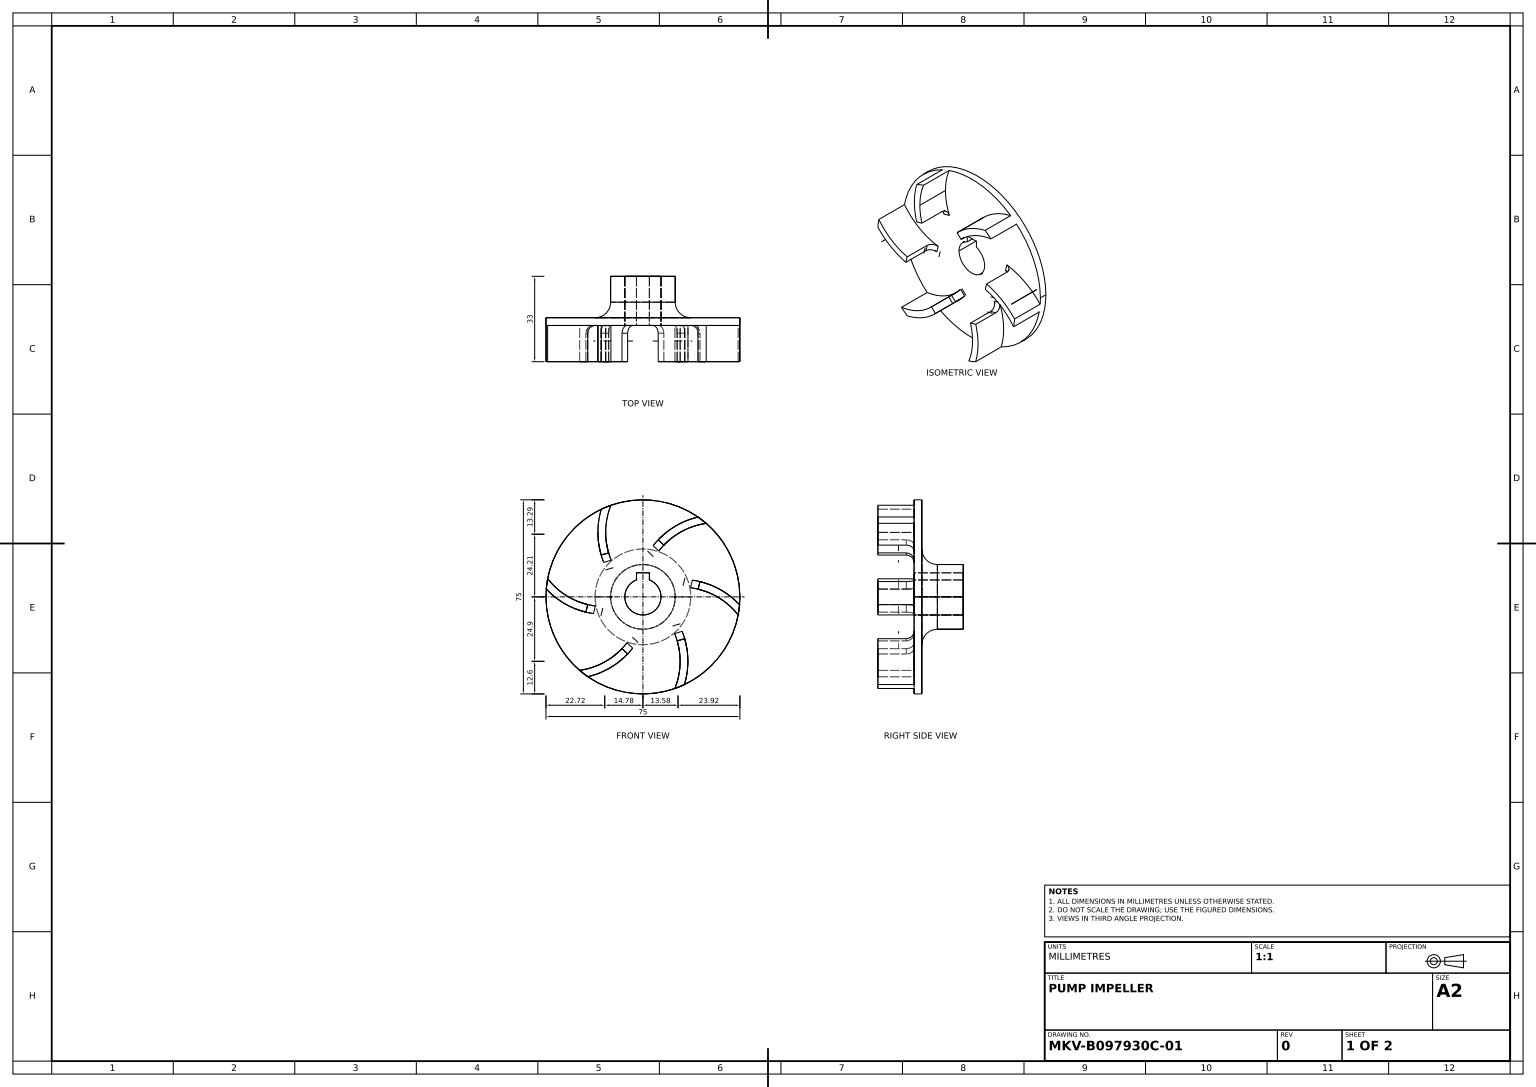
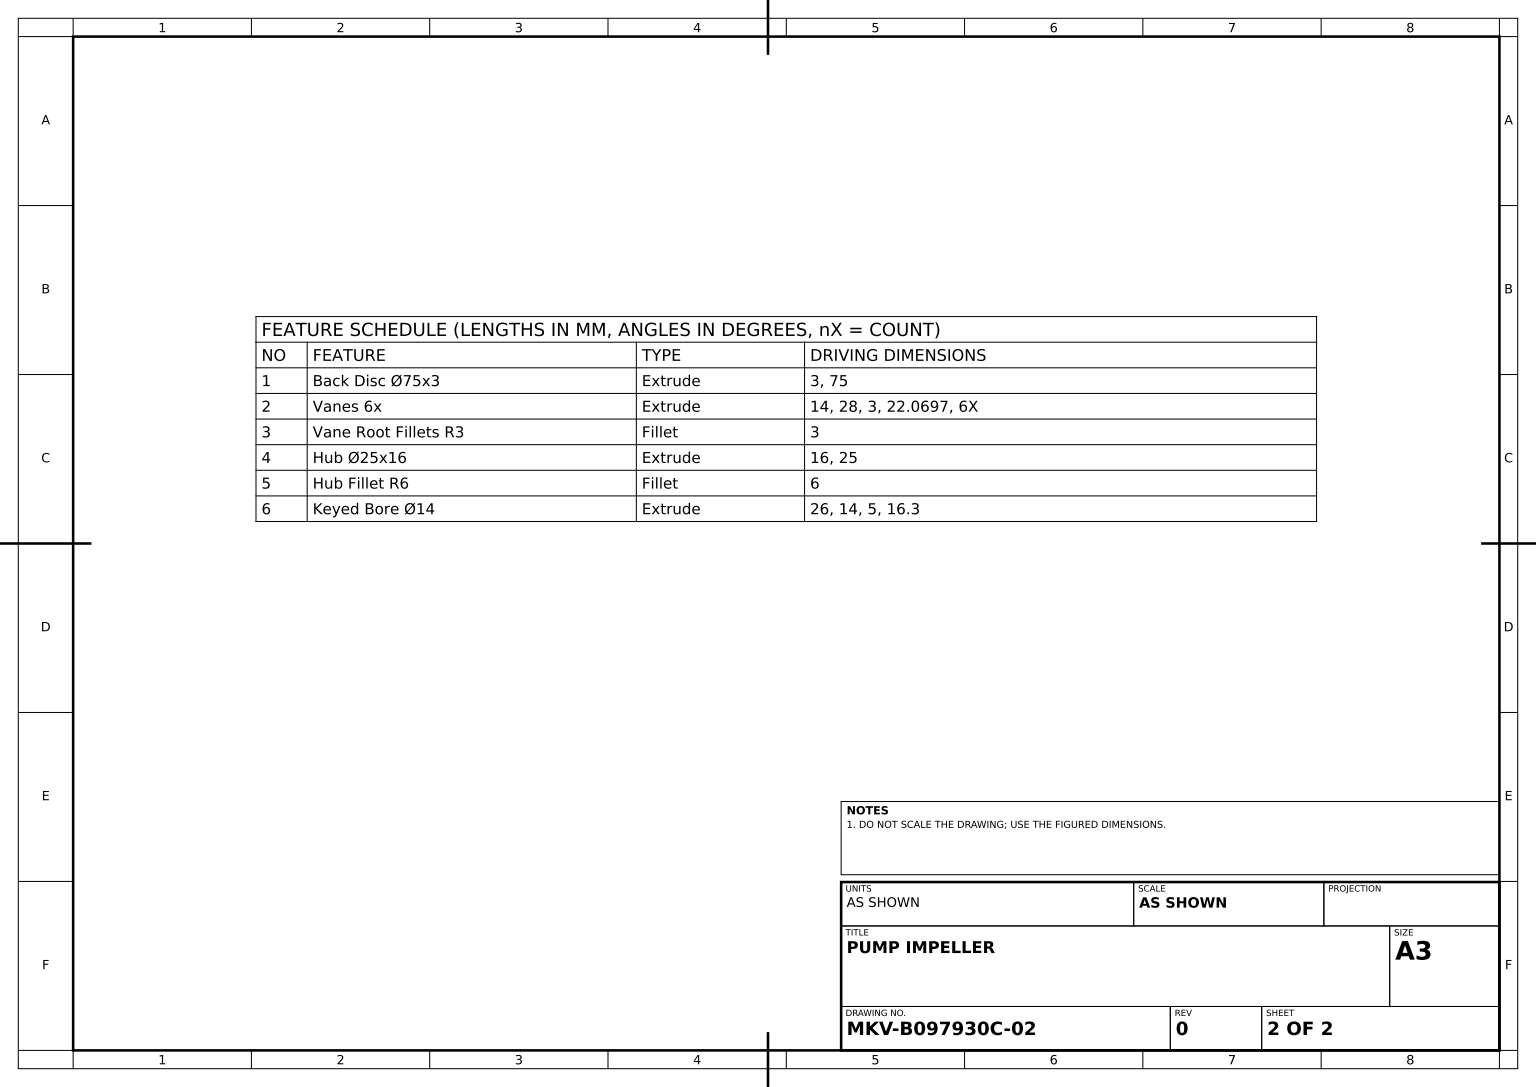
from build123d import *
from build123d.topology import SkipClean

# Parameters (mm, degrees)
BACK_DISC_SKETCH_75_R  = 37.5
BACK_DISC_75X3_DEPTH   = 3
VANES_6X_DEPTH         = 14
VANE_ROOT_FILLETS_R3_R = 3
HUB_SKETCH_25_R        = 12.5
HUB_25X16_DEPTH        = 16
HUB_FILLET_R6_R        = 6
KEYED_BORE_14_DEPTH    = 26


with BuildPart() as part:
    # Back Disc Sketch Ø75 → Back Disc Ø75x3 (new body)
    with BuildSketch(Plane.XY):
        Circle(BACK_DISC_SKETCH_75_R)
    extrude(amount=BACK_DISC_75X3_DEPTH)

    # Vane Profiles 6x Sketch → Vanes 6x (add)
    with SkipClean():  # the faces are left unmerged after this step: merging them gives an invalid solid
        with BuildSketch(Plane.XY.offset(3)):
            with BuildLine():
                Line((-21.363742831, -3), (-22.069677344, -5.915760015))
                ThreePointArc((-22.069677344, -5.915760015), (-30.375240954, -2.574915234), (-37.379807383, 3))
                ThreePointArc((-37.379807383, 3), (-37.165438921, 4.998014583), (-36.844350715, 6.981677477))
                ThreePointArc((-36.844350715, 6.981677477), (-29.948334758, 0.681430448), (-21.363742831, -3))
            make_face()
            with BuildLine():
                Line((-13.279947627, 17.001544011), (-16.158037127, 16.155021226))
                ThreePointArc((-16.158037127, 16.155021226), (-17.417562483, 25.018272695), (-16.09182748, 33.871862782))
                ThreePointArc((-16.09182748, 33.871862782), (-14.254311863, 34.68522154), (-12.375865302, 35.398982443))
                ThreePointArc((-12.375865302, 35.398982443), (-14.384031301, 26.276733925), (-13.279947627, 17.001544011))
            make_face()
            with BuildLine():
                Line((8.083795204, 20.001544011), (5.911640217, 22.070781241))
                ThreePointArc((5.911640217, 22.070781241), (12.957678472, 27.59318793), (21.287979903, 30.871862782))
                ThreePointArc((21.287979903, 30.871862782), (22.911127058, 29.687206957), (24.468485413, 28.417304967))
                ThreePointArc((24.468485413, 28.417304967), (15.564303458, 25.595303478), (8.083795204, 20.001544011))
            make_face()
            with BuildLine():
                Line((21.363742831, 3), (22.069677344, 5.915760015))
                ThreePointArc((22.069677344, 5.915760015), (30.375240954, 2.574915234), (37.379807383, -3))
                ThreePointArc((37.379807383, -3), (37.165438921, -4.998014583), (36.844350715, -6.981677477))
                ThreePointArc((36.844350715, -6.981677477), (29.948334758, -0.681430448), (21.363742831, 3))
            make_face()
            with BuildLine():
                Line((13.279947627, -17.001544011), (16.158037127, -16.155021226))
                ThreePointArc((16.158037127, -16.155021226), (17.417562483, -25.018272695), (16.09182748, -33.871862782))
                ThreePointArc((16.09182748, -33.871862782), (14.254311863, -34.68522154), (12.375865302, -35.398982443))
                ThreePointArc((12.375865302, -35.398982443), (14.384031301, -26.276733925), (13.279947627, -17.001544011))
            make_face()
            with BuildLine():
                Line((-8.083795204, -20.001544011), (-5.911640217, -22.070781241))
                ThreePointArc((-5.911640217, -22.070781241), (-12.957678472, -27.59318793), (-21.287979903, -30.871862782))
                ThreePointArc((-21.287979903, -30.871862782), (-22.911127058, -29.687206957), (-24.468485413, -28.417304967))
                ThreePointArc((-24.468485413, -28.417304967), (-15.564303458, -25.595303478), (-8.083795204, -20.001544011))
            make_face()
        extrude(amount=VANES_6X_DEPTH)

    # Vane Root Fillets R3
    vane_root_fillets_r3_edges = [part.edges().sort_by_distance(p)[0] for p in [
        (-14.718992377, 16.578282619, 3),
        (6.99771771, 21.036162626, 3),
        (21.716710087, 4.457880007, 3),
        (14.718992377, -16.578282619, 3),
        (-6.99771771, -21.036162626, 3),
        (-21.716710087, -4.457880007, 3),
    ]]
    fillet(vane_root_fillets_r3_edges, radius=VANE_ROOT_FILLETS_R3_R)

    # Hub Sketch Ø25 → Hub Ø25x16 (add)
    with SkipClean():  # the faces are left unmerged after this step: merging them gives an invalid solid
        with BuildSketch(Plane(origin=(0, 0, 0), x_dir=(-1, 0, 0), z_dir=(0, 0, -1))):
            Circle(HUB_SKETCH_25_R)
        extrude(amount=HUB_25X16_DEPTH)

    # Hub Fillet R6
    hub_fillet_r6_edges = [part.edges().sort_by_distance(p)[0] for p in [
        (12.5, 0, 0),
    ]]
    fillet(hub_fillet_r6_edges, radius=HUB_FILLET_R6_R)

    # Keyed Bore Sketch Ø14 → Keyed Bore Ø14 (cut)
    with SkipClean():  # the faces are left unmerged after this step: merging them gives an invalid solid
        with BuildSketch(Plane.XY.offset(3)):
            with BuildLine():
                Line((-2.5, 9.3), (2.5, 9.3))
                Line((2.5, 9.3), (2.5, 6.538348415))
                ThreePointArc((2.5, 6.538348415), (0, -7), (-2.5, 6.538348415))
                Line((-2.5, 6.538348415), (-2.5, 9.3))
            make_face()
        extrude(amount=-KEYED_BORE_14_DEPTH, mode=Mode.SUBTRACT)


solid = part.part
